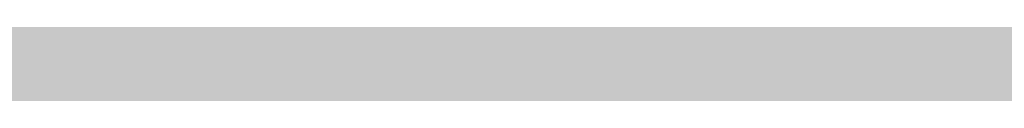
# Model space of a CAD drawing. Units: millimetres. Extents: x 0 to 2267, y 0 to 1823.
# Tile 178 of 256: x 1838.83 to 1841.442, y 1127.15 to 1127.306. Entities that reach past the tile are written whole.
import ezdxf

# ---------------------------------------------------------------- set-up
doc = ezdxf.new("R2010")
doc.units = ezdxf.units.MM
doc.header["$MEASUREMENT"] = 0
doc.layers.add('M-DIMS', color=2, linetype='Continuous', lineweight=25)
doc.layers.add('M-HATC', color=252, linetype='Continuous', lineweight=18)
doc.styles.get("Standard").update_dxf_attribs({"font": 'arial.ttf'})
doc.dimstyles.get("Standard").update_dxf_attribs({"dimtxt": 7, "dimasz": 4, "dimexe": 0.18, "dimexo": 0.0625, "dimgap": 0.09, "dimtad": 0, "dimdec": 0, "dimzin": 0, "dimdsep": 46, "dimtxsty": 'Standard', "dimcen": 0.09, "dimadec": 0, "dimazin": 0, "dimtfac": 1, "dimtdec": 0, "dimtofl": 0, "dimtmove": 0, "dimatfit": 3, "dimfxl": 1, "dimtolj": 1, "dimtzin": 0, "dimarcsym": 0})

# ---------------------------------------------------------------- blocks, each defined once
blk = doc.blocks.new('*D1')
at = {"layer": 'Defpoints', "color": 0, "transparency": 16777216}
for p in [(1593.4289, 1127.4171), (1843.4289, 1127.4171), (1843.4289, 955.6278)]:
    blk.add_point(p, dxfattribs=at)
at = {"layer": 'M-DIMS', "color": 0, "lineweight": -2, "transparency": 16777216}
for p, q in [((1593.4289, 1127.3546), (1593.4289, 955.4478)), ((1843.4289, 1127.3546), (1843.4289, 955.4478)), ((1597.4289, 955.6278), (1710.5582, 955.6278)), ((1839.4289, 955.6278), (1726.2996, 955.6278))]:
    blk.add_line(p, q, dxfattribs=at)
at = {"layer": 'M-DIMS', "color": 0, "transparency": 16777216}
for points in [[(1597.4289, 956.2944), (1597.4289, 954.9611), (1593.4289, 955.6278)], [(1839.4289, 956.2944), (1839.4289, 954.9611), (1843.4289, 955.6278)]]:
    blk.add_solid(points, dxfattribs=at)
at = {"layer": 'M-DIMS', "color": 0, "transparency": 16777216, "insert": (1718.4289, 955.6278), "char_height": 7, "attachment_point": 5}
blk.add_mtext('\\A1;250', dxfattribs=at)

msp = doc.modelspace()

# ---------------------------------------------------------------- hatches: boundary and pattern name
at = {"layer": 'M-HATC'}
h = msp.add_hatch(color=256, dxfattribs=at)
h.dxf.hatch_style = 1
h.paths.add_polyline_path([(2055.771, 1603.062), (1381.0868, 1603.062), (1381.0868, 1598.062), (2055.771, 1598.062)])
h.paths.add_polyline_path([(2055.771, 1598.062), (1381.0868, 1598.062), (1381.0868, 1593.062), (2055.771, 1593.062)])
h.paths.add_polyline_path([(2051.3074, 1536.7609), (1385.5504, 1536.7609), (1385.5504, 1526.7609), (1387.5504, 1526.7609), (1388.5366, 1525.0528), (1385.3319, 1521.2335), (1385.3319, 1521.2226), (2050.2542, 1522.7491), (2048.3212, 1525.0528), (2049.3074, 1526.7609), (2051.3074, 1526.7609)])
edge = h.paths.add_edge_path()
edge.add_arc((1847.5345, 1379.1492), 135, 222.603061, 222.890851, ccw=False)
edge.add_line((1748.1663, 1287.7656), (1683.0921, 1287.7656))
edge.add_arc((1583.7239, 1379.1492), 135, 317.109149, 317.396939, ccw=False)
edge.add_arc((1678.9686, 1290.6707), 5, 222.8909, 317.1091, ccw=False)
edge.add_arc((1774.2133, 1379.1492), 135, 222.603061, 222.890851, ccw=False)
edge.add_line((1674.8451, 1287.7656), (1609.7709, 1287.7656))
edge.add_arc((1510.4027, 1379.1492), 135, 317.109149, 317.396939, ccw=False)
edge.add_arc((1605.6474, 1290.6707), 5, 222.8909, 317.1091, ccw=False)
edge.add_arc((1700.8921, 1379.1492), 135, 222.603061, 222.890851, ccw=False)
edge.add_line((1601.5239, 1287.7656), (1536.4497, 1287.7656))
edge.add_arc((1437.0815, 1379.1492), 135, 317.109149, 317.396939, ccw=False)
edge.add_arc((1532.3262, 1290.6707), 5, 222.8909, 317.1091, ccw=False)
edge.add_arc((1627.5709, 1379.1492), 135, 222.603061, 222.890851, ccw=False)
edge.add_line((1528.2027, 1287.7656), (1505.9289, 1287.7656))
edge.add_spline(control_points=[(1505.9289, 1287.7656), (1504.2622, 1287.7656), (1504.2622, 1282.7656), (1505.9289, 1282.7656)], knot_values=[0, 0, 0, 0, 5, 5, 5, 5], degree=3, periodic=0)
edge.add_line((1505.9289, 1282.7656), (1930.9289, 1282.7656))
edge.add_spline(control_points=[(1930.9289, 1282.7656), (1932.5956, 1282.7656), (1932.5956, 1287.7656), (1930.9289, 1287.7656)], knot_values=[0, 0, 0, 0, 5, 5, 5, 5], degree=3, periodic=0)
edge.add_line((1930.9289, 1287.7656), (1903.0557, 1287.7656))
edge.add_arc((1803.6875, 1379.1492), 135, 317.109149, 317.396939, ccw=False)
edge.add_arc((1898.9322, 1290.6707), 5, 222.8909, 317.1091, ccw=False)
edge.add_arc((1994.1769, 1379.1492), 135, 222.603061, 222.890851, ccw=False)
edge.add_line((1894.8087, 1287.7656), (1829.7345, 1287.7656))
edge.add_arc((1730.3663, 1379.1492), 135, 317.109149, 317.396939, ccw=False)
edge.add_arc((1825.611, 1290.6707), 5, 222.8909, 317.1091, ccw=False)
edge.add_arc((1920.8557, 1379.1492), 135, 222.603061, 222.890851, ccw=False)
edge.add_line((1821.4875, 1287.7656), (1756.4133, 1287.7656))
edge.add_arc((1657.0451, 1379.1492), 135, 317.109149, 317.396939, ccw=False)
edge.add_arc((1752.2898, 1290.6707), 5, 222.8909, 317.1091, ccw=False)
edge = h.paths.add_edge_path()
edge.add_spline(control_points=[(1843.4289, 1227.2475), (1845.0956, 1227.2475), (1845.0956, 1232.2475), (1843.4289, 1232.2475)], knot_values=[0, 0, 0, 0, 5, 5, 5, 5], degree=3, periodic=0)
edge.add_line((1843.4289, 1232.2475), (1593.4289, 1232.2475))
edge.add_spline(control_points=[(1593.4289, 1232.2475), (1591.7622, 1232.2475), (1591.7622, 1227.2475), (1593.4289, 1227.2475)], knot_values=[0, 0, 0, 0, 5, 5, 5, 5], degree=3, periodic=0)
edge.add_line((1593.4289, 1227.2475), (1843.4289, 1227.2475))
h.paths.add_polyline_path([(1905.9289, 1127.4171), (1530.9289, 1127.4171, 0.414214), (1520.9289, 1117.4171), (1530.9289, 1117.4171), (1915.9289, 1117.4171, 0.414214)])
edge = h.paths.add_edge_path()
edge.add_arc((1397.0858, 1498.4078), 12.7299, 90.78215, 190.87871, ccw=False)
edge.add_line((1396.912, 1511.1365), (1428.0097, 1511.3488))
edge.add_line((1428.0097, 1511.3488), (1433.0097, 1511.3488))
edge.add_line((1433.0097, 1511.3488), (1434.439, 1511.3488))
edge.add_arc((1419.474, 1498.0804), 20, 41.561, 74.08211)
edge.add_line((1424.9592, 1517.3135), (1399.9351, 1517.2561))
edge.add_spline(control_points=[(1399.9307, 1517.2561), (1399.884, 1517.2131), (1399.8328, 1517.1689), (1399.7774, 1517.1236)], knot_values=[11.567499, 11.567499, 11.567499, 11.567499, 11.814249, 11.814249, 11.814249, 11.814249], degree=3, periodic=0)
edge.add_spline(control_points=[(1399.6328, 1517.0099), (1399.5831, 1516.9721), (1399.5307, 1516.9338), (1399.4759, 1516.8947)], knot_values=[11.167718, 11.167718, 11.167718, 11.167718, 11.365188, 11.365188, 11.365188, 11.365188], degree=3, periodic=0)
edge.add_spline(control_points=[(1399.3398, 1516.8001), (1399.1514, 1516.6719), (1398.9384, 1516.5377), (1398.704, 1516.3994)], knot_values=[10.376405, 10.376405, 10.376405, 10.376405, 11.00994, 11.00994, 11.00994, 11.00994], degree=3, periodic=0)
edge.add_spline(control_points=[(1398.6572, 1516.3719), (1398.5789, 1516.326), (1398.4983, 1516.2797), (1398.4155, 1516.2331)], knot_values=[10.125175, 10.125175, 10.125175, 10.125175, 10.334406, 10.334406, 10.334406, 10.334406], degree=3, periodic=0)
edge.add_spline(control_points=[(1398.2642, 1516.1487), (1398.196, 1516.1111), (1398.1263, 1516.0732), (1398.0555, 1516.0351)], knot_values=[9.832246, 9.832246, 9.832246, 9.832246, 9.999658, 9.999658, 9.999658, 9.999658], degree=3, periodic=0)
edge.add_spline(control_points=[(1397.9987, 1516.0048), (1397.7312, 1515.8621), (1397.446, 1515.7171), (1397.1466, 1515.5714)], knot_values=[9.161808, 9.161808, 9.161808, 9.161808, 9.787769, 9.787769, 9.787769, 9.787769], degree=3, periodic=0)
edge.add_spline(control_points=[(1397.1466, 1515.5714), (1396.8418, 1515.423), (1396.5222, 1515.274), (1396.1914, 1515.1262)], knot_values=[8.524455, 8.524455, 8.524455, 8.524455, 9.161808, 9.161808, 9.161808, 9.161808], degree=3, periodic=0)
edge.add_spline(control_points=[(1396.0777, 1515.0756), (1395.9854, 1515.0348), (1395.8922, 1514.994), (1395.7983, 1514.9534)], knot_values=[8.275193, 8.275193, 8.275193, 8.275193, 8.451726, 8.451726, 8.451726, 8.451726], degree=3, periodic=0)
edge.add_spline(control_points=[(1395.6018, 1514.8691), (1395.4997, 1514.8257), (1395.3968, 1514.7824), (1395.2932, 1514.7394)], knot_values=[7.962917, 7.962917, 7.962917, 7.962917, 8.152764, 8.152764, 8.152764, 8.152764], degree=3, periodic=0)
edge.add_spline(control_points=[(1395.2116, 1514.7057), (1394.8278, 1514.5475), (1394.4345, 1514.3929), (1394.0364, 1514.2442)], knot_values=[7.21254, 7.21254, 7.21254, 7.21254, 7.913148, 7.913148, 7.913148, 7.913148], degree=3, periodic=0)
edge.add_spline(control_points=[(1394.0364, 1514.2442), (1393.7076, 1514.1214), (1393.3754, 1514.0027), (1393.0427, 1513.8895)], knot_values=[6.633733, 6.633733, 6.633733, 6.633733, 7.21254, 7.21254, 7.21254, 7.21254], degree=3, periodic=0)
edge.add_spline(control_points=[(1392.8214, 1513.815), (1392.7198, 1513.7812), (1392.6181, 1513.7479), (1392.5166, 1513.7152)], knot_values=[6.328796, 6.328796, 6.328796, 6.328796, 6.505493, 6.505493, 6.505493, 6.505493], degree=3, periodic=0)
edge.add_spline(control_points=[(1392.5166, 1513.7152), (1392.3187, 1513.6515), (1392.1212, 1513.59), (1391.9244, 1513.531)], knot_values=[5.984605, 5.984605, 5.984605, 5.984605, 6.328796, 6.328796, 6.328796, 6.328796], degree=3, periodic=0)
edge.add_spline(control_points=[(1391.7915, 1513.4915), (1391.3122, 1513.3501), (1390.8384, 1513.2239), (1390.3784, 1513.1171)], knot_values=[5.066697, 5.066697, 5.066697, 5.066697, 5.907055, 5.907055, 5.907055, 5.907055], degree=3, periodic=0)
edge.add_spline(control_points=[(1390.3784, 1513.1171), (1390.1797, 1513.071), (1389.9836, 1513.0284), (1389.7907, 1512.9899)], knot_values=[4.70367, 4.70367, 4.70367, 4.70367, 5.066695, 5.066695, 5.066695, 5.066695], degree=3, periodic=0)
edge.add_spline(control_points=[(1389.422, 1512.9204), (1389.2459, 1512.8892), (1389.0729, 1512.8617), (1388.9036, 1512.8381)], knot_values=[4.130571, 4.130571, 4.130571, 4.130571, 4.469816, 4.469816, 4.469816, 4.469816], degree=3, periodic=0)
edge.add_spline(control_points=[(1388.9036, 1512.8381), (1388.591, 1512.7946), (1388.2911, 1512.7644), (1388.0071, 1512.7494)], knot_values=[3.504031, 3.504031, 3.504031, 3.504031, 4.130571, 4.130571, 4.130571, 4.130571], degree=3, periodic=0)
edge.add_spline(control_points=[(1387.9356, 1512.7459), (1387.8538, 1512.7423), (1387.7733, 1512.74), (1387.6944, 1512.739)], knot_values=[3.268866, 3.268866, 3.268866, 3.268866, 3.451164, 3.451164, 3.451164, 3.451164], degree=3, periodic=0)
edge.add_spline(control_points=[(1387.3351, 1512.7443), (1387.2076, 1512.7499), (1387.0847, 1512.7597), (1386.967, 1512.7739)], knot_values=[2.670686, 2.670686, 2.670686, 2.670686, 2.984, 2.984, 2.984, 2.984], degree=3, periodic=0)
edge.add_spline(control_points=[(1386.8327, 1512.7922), (1386.8209, 1512.7941), (1386.8092, 1512.7959), (1386.7975, 1512.7979)], knot_values=[2.516981, 2.516981, 2.516981, 2.516981, 2.549528, 2.549528, 2.549528, 2.549528], degree=3, periodic=0)
edge.add_spline(control_points=[(1386.4526, 1512.8735), (1386.4257, 1512.881), (1386.3993, 1512.889), (1386.3733, 1512.8972)], knot_values=[2.095869, 2.095869, 2.095869, 2.095869, 2.17941, 2.17941, 2.17941, 2.17941], degree=3, periodic=0)
edge.add_spline(control_points=[(1386.0691, 1513.0189), (1386.0634, 1513.0217), (1386.0577, 1513.0246), (1386.052, 1513.0275)], knot_values=[1.72453, 1.72453, 1.72453, 1.72453, 1.745933, 1.745933, 1.745933, 1.745933], degree=3, periodic=0)
edge.add_arc((1399.474, 1498.0804), 20, 131.82432, 180)
edge.add_arc((1630.3336, 1505.5484), 250.9708, 181.705176, 236.427975)
edge.add_arc((1605.3399, 1483.3044), 218.7822, 238.660829, 243.34961)
edge.add_arc((1647.0911, 1510.3592), 262.8986, 183.129836, 237.853442, ccw=False)
h.paths.add_polyline_path([(1406.5369, 1391.9644, 0.149382), (1491.5506, 1296.4418, -0.129517)], flags=17)
edge = h.paths.add_edge_path()
edge.add_arc((2037.3838, 1498.0804), 20, 0, 48.26587)
edge.add_spline(control_points=[(2050.6973, 1513.0052), (2050.6512, 1512.9847), (2050.6034, 1512.9655), (2050.5539, 1512.9477)], knot_values=[1.835652, 1.835652, 1.835652, 1.835652, 2.000781, 2.000781, 2.000781, 2.000781], degree=3, periodic=0)
edge.add_spline(control_points=[(2050.4616, 1512.9166), (2050.479, 1512.9221), (2050.4963, 1512.9277), (2050.5133, 1512.9335)], knot_values=[2.045477, 2.045477, 2.045477, 2.045477, 2.101389, 2.101389, 2.101389, 2.101389], degree=3, periodic=0)
edge.add_spline(control_points=[(2050.129, 1512.8342), (2050.1984, 1512.8473), (2050.2657, 1512.8623), (2050.3308, 1512.8792)], knot_values=[2.237629, 2.237629, 2.237629, 2.237629, 2.435841, 2.435841, 2.435841, 2.435841], degree=3, periodic=0)
edge.add_spline(control_points=[(2050.0946, 1512.8278), (2050.1061, 1512.8299), (2050.1176, 1512.832), (2050.129, 1512.8342)], knot_values=[2.435841, 2.435841, 2.435841, 2.435841, 2.468321, 2.468321, 2.468321, 2.468321], degree=3, periodic=0)
edge.add_spline(control_points=[(2049.7843, 1512.7851), (2049.8552, 1512.7922), (2049.9243, 1512.8008), (2049.9917, 1512.8109)], knot_values=[2.563852, 2.563852, 2.563852, 2.563852, 2.748541, 2.748541, 2.748541, 2.748541], degree=3, periodic=0)
edge.add_spline(control_points=[(2049.4052, 1512.7617), (2049.5364, 1512.7653), (2049.6629, 1512.773), (2049.7843, 1512.7851)], knot_values=[2.748541, 2.748541, 2.748541, 2.748541, 3.064882, 3.064882, 3.064882, 3.064882], degree=3, periodic=0)
edge.add_spline(control_points=[(2049.1698, 1512.7597), (2049.2336, 1512.7591), (2049.2965, 1512.7594), (2049.3584, 1512.7606)], knot_values=[3.102309, 3.102309, 3.102309, 3.102309, 3.2503, 3.2503, 3.2503, 3.2503], degree=3, periodic=0)
edge.add_spline(control_points=[(2048.8573, 1512.7691), (2048.9638, 1512.7638), (2049.068, 1512.7606), (2049.1698, 1512.7597)], knot_values=[3.2503, 3.2503, 3.2503, 3.2503, 3.486069, 3.486069, 3.486069, 3.486069], degree=3, periodic=0)
edge.add_spline(control_points=[(2048.6924, 1512.7789), (2048.3729, 1512.8009), (2048.0345, 1512.8411), (2047.6817, 1512.897)], knot_values=[3.606429, 3.606429, 3.606429, 3.606429, 4.2989, 4.2989, 4.2989, 4.2989], degree=3, periodic=0)
edge.add_spline(control_points=[(2047.6817, 1512.897), (2047.5458, 1512.9185), (2047.4077, 1512.9424), (2047.2678, 1512.9685)], knot_values=[4.2989, 4.2989, 4.2989, 4.2989, 4.565769, 4.565769, 4.565769, 4.565769], degree=3, periodic=0)
edge.add_spline(control_points=[(2047.2678, 1512.9685), (2047.1449, 1512.9914), (2047.0207, 1513.016), (2046.8951, 1513.0422)], knot_values=[4.565769, 4.565769, 4.565769, 4.565769, 4.799971, 4.799971, 4.799971, 4.799971], degree=3, periodic=0)
edge.add_spline(control_points=[(2046.8951, 1513.0422), (2046.5286, 1513.1188), (2046.1513, 1513.209), (2045.7676, 1513.3107)], knot_values=[4.799971, 4.799971, 4.799971, 4.799971, 5.483718, 5.483718, 5.483718, 5.483718], degree=3, periodic=0)
edge.add_spline(control_points=[(2045.7676, 1513.3107), (2045.3724, 1513.4154), (2044.9704, 1513.5322), (2044.5662, 1513.6588)], knot_values=[5.483718, 5.483718, 5.483718, 5.483718, 6.187866, 6.187866, 6.187866, 6.187866], degree=3, periodic=0)
edge.add_spline(control_points=[(2044.5662, 1513.6588), (2044.4149, 1513.7061), (2044.2633, 1513.7549), (2044.1116, 1513.8048)], knot_values=[6.187866, 6.187866, 6.187866, 6.187866, 6.451551, 6.451551, 6.451551, 6.451551], degree=3, periodic=0)
edge.add_spline(control_points=[(2044.1116, 1513.8048), (2043.9967, 1513.8427), (2043.8817, 1513.8813), (2043.7668, 1513.9205)], knot_values=[6.451551, 6.451551, 6.451551, 6.451551, 6.651434, 6.651434, 6.651434, 6.651434], degree=3, periodic=0)
edge.add_spline(control_points=[(2043.7668, 1513.9205), (2043.3716, 1514.0554), (2042.9774, 1514.1979), (2042.5886, 1514.3458)], knot_values=[6.651434, 6.651434, 6.651434, 6.651434, 7.338879, 7.338879, 7.338879, 7.338879], degree=3, periodic=0)
edge.add_spline(control_points=[(2042.5886, 1514.3458), (2042.1643, 1514.5071), (2041.7465, 1514.6749), (2041.3409, 1514.846)], knot_values=[7.338879, 7.338879, 7.338879, 7.338879, 8.089209, 8.089209, 8.089209, 8.089209], degree=3, periodic=0)
edge.add_spline(control_points=[(2041.3409, 1514.846), (2041.1028, 1514.9465), (2040.869, 1515.0481), (2040.6405, 1515.1502)], knot_values=[8.089209, 8.089209, 8.089209, 8.089209, 8.529587, 8.529587, 8.529587, 8.529587], degree=3, periodic=0)
edge.add_spline(control_points=[(2040.51, 1515.2089), (2040.0824, 1515.4022), (2039.6747, 1515.5971), (2039.295, 1515.7894)], knot_values=[8.613818, 8.613818, 8.613818, 8.613818, 9.44571, 9.44571, 9.44571, 9.44571], degree=3, periodic=0)
edge.add_spline(control_points=[(2039.295, 1515.7894), (2039.0618, 1515.9075), (2038.8391, 1516.0246), (2038.6288, 1516.1398)], knot_values=[9.44571, 9.44571, 9.44571, 9.44571, 9.956404, 9.956404, 9.956404, 9.956404], degree=3, periodic=0)
edge.add_spline(control_points=[(2038.6288, 1516.1398), (2038.5187, 1516.2001), (2038.4121, 1516.2598), (2038.309, 1516.3189)], knot_values=[9.956404, 9.956404, 9.956404, 9.956404, 10.223542, 10.223542, 10.223542, 10.223542], degree=3, periodic=0)
edge.add_spline(control_points=[(2038.309, 1516.3189), (2038.2138, 1516.3735), (2038.1216, 1516.4276), (2038.0328, 1516.481)], knot_values=[10.223542, 10.223542, 10.223542, 10.223542, 10.47051, 10.47051, 10.47051, 10.47051], degree=3, periodic=0)
edge.add_spline(control_points=[(2038.0328, 1516.481), (2037.7855, 1516.6296), (2037.5639, 1516.773), (2037.3722, 1516.909)], knot_values=[10.47051, 10.47051, 10.47051, 10.47051, 11.15767, 11.15767, 11.15767, 11.15767], degree=3, periodic=0)
edge.add_spline(control_points=[(2037.3722, 1516.909), (2037.2789, 1516.9752), (2037.1927, 1517.0396), (2037.1142, 1517.102)], knot_values=[11.15767, 11.15767, 11.15767, 11.15767, 11.49227, 11.49227, 11.49227, 11.49227], degree=3, periodic=0)
edge.add_spline(control_points=[(2036.8564, 1517.3259), (2036.9148, 1517.2692), (2036.9814, 1517.2103), (2037.0557, 1517.1492)], knot_values=[11.577341, 11.577341, 11.577341, 11.577341, 11.91035, 11.91035, 11.91035, 11.91035], degree=3, periodic=0)
edge.add_spline(control_points=[(2036.8074, 1517.3748), (2036.823, 1517.3587), (2036.8393, 1517.3424), (2036.8564, 1517.3259)], knot_values=[11.91035, 11.91035, 11.91035, 11.91035, 12.007402, 12.007402, 12.007402, 12.007402], degree=3, periodic=0)
edge.add_spline(control_points=[(2036.7017, 1517.494), (2036.7104, 1517.483), (2036.7196, 1517.4719), (2036.7291, 1517.4606)], knot_values=[12.184155, 12.184155, 12.184155, 12.184155, 12.255409, 12.255409, 12.255409, 12.255409], degree=3, periodic=0)
edge.add_spline(control_points=[(2036.6159, 1517.6205), (2036.62, 1517.613), (2036.6243, 1517.6055), (2036.6289, 1517.5979)], knot_values=[12.487913, 12.487913, 12.487913, 12.487913, 12.541035, 12.541035, 12.541035, 12.541035], degree=3, periodic=0)
edge.add_spline(control_points=[(2036.5635, 1517.786), (2036.5637, 1517.7794), (2036.5642, 1517.7726), (2036.565, 1517.7658)], knot_values=[12.911761, 12.911761, 12.911761, 12.911761, 12.968286, 12.968286, 12.968286, 12.968286], degree=3, periodic=0)
edge.add_spline(control_points=[(2036.6166, 1517.9304), (2036.6125, 1517.9259), (2036.6086, 1517.9212), (2036.6049, 1517.9165)], knot_values=[13.382527, 13.382527, 13.382527, 13.382527, 13.433791, 13.433791, 13.433791, 13.433791], degree=3, periodic=0)
edge.add_spline(control_points=[(2036.749, 1518.017), (2036.7361, 1518.0116), (2036.7239, 1518.006), (2036.7124, 1518.0002)], knot_values=[13.726299, 13.726299, 13.726299, 13.726299, 13.809928, 13.809928, 13.809928, 13.809928], degree=3, periodic=0)
edge.add_spline(control_points=[(2036.8604, 1518.0528), (2036.8386, 1518.0474), (2036.8181, 1518.0416), (2036.7988, 1518.0353)], knot_values=[13.910887, 13.910887, 13.910887, 13.910887, 14.02153, 14.02153, 14.02153, 14.02153], degree=3, periodic=0)
edge.add_line((2036.9639, 1518.0804), (2032.3838, 1518.0804))
edge.add_line((2032.3838, 1518.0804), (2027.3838, 1518.0804))
edge.add_line((2027.3838, 1518.0804), (2022.3838, 1518.0804))
edge.add_line((2022.3838, 1518.0804), (2017.3838, 1518.0804))
edge.add_arc((2017.3838, 1498.0804), 20, 90, 138.439)
edge.add_line((2002.4188, 1511.3488), (2003.8481, 1511.3488))
edge.add_line((2003.8481, 1511.3488), (2008.8481, 1511.3488))
edge.add_line((2008.8481, 1511.3488), (2039.772, 1511.1377))
edge.add_arc((2039.772, 1498.4078), 12.7299, -10.87871, 90, ccw=False)
edge.add_arc((1789.7668, 1510.3592), 262.8986, 302.146558, 356.870164, ccw=False)
edge.add_arc((1831.5179, 1483.3044), 218.7822, 296.65039, 301.339171)
edge.add_arc((1806.5242, 1505.5484), 250.9708, 303.572025, 358.294824)
h.paths.add_polyline_path([(2030.321, 1391.9644, -0.129517), (1945.3072, 1296.4418, 0.149382)], flags=17)
edge = h.paths.add_edge_path()
edge.add_spline(control_points=[(2037.2464, 1518.0821), (2037.2898, 1518.081), (2037.3355, 1518.0804), (2037.3838, 1518.0804)], knot_values=[0.000012, 0.000012, 0.000012, 0.000012, 0.144754, 0.144754, 0.144754, 0.144754], degree=3, periodic=0)
edge.add_line((2037.3357, 1518.0804), (2037.0096, 1518.0804))
edge.add_spline(control_points=[(2037.0096, 1518.0804), (2036.9822, 1518.0768), (2036.956, 1518.0727), (2036.9312, 1518.0681)], knot_values=[14.13465, 14.13465, 14.13465, 14.13465, 14.247197, 14.247197, 14.247197, 14.247197], degree=3, periodic=0)
edge.add_spline(control_points=[(2036.9312, 1518.0681), (2036.9276, 1518.0674), (2036.9241, 1518.0667), (2036.9205, 1518.0661)], knot_values=[14.118315, 14.118315, 14.118315, 14.118315, 14.13465, 14.13465, 14.13465, 14.13465], degree=3, periodic=0)
edge.add_spline(control_points=[(2036.9205, 1518.0661), (2036.9118, 1518.0644), (2036.9032, 1518.0626), (2036.8948, 1518.0608)], knot_values=[14.078086, 14.078086, 14.078086, 14.078086, 14.118315, 14.118315, 14.118315, 14.118315], degree=3, periodic=0)
edge.add_spline(control_points=[(2036.8948, 1518.0608), (2036.883, 1518.0583), (2036.8716, 1518.0556), (2036.8604, 1518.0528)], knot_values=[14.02153, 14.02153, 14.02153, 14.02153, 14.078086, 14.078086, 14.078086, 14.078086], degree=3, periodic=0)
edge.add_spline(control_points=[(2036.8604, 1518.0528), (2036.8386, 1518.0474), (2036.8181, 1518.0416), (2036.7988, 1518.0353)], knot_values=[13.910887, 13.910887, 13.910887, 13.910887, 14.02153, 14.02153, 14.02153, 14.02153], degree=3, periodic=0)
edge.add_spline(control_points=[(2036.7988, 1518.0353), (2036.7981, 1518.035), (2036.7974, 1518.0348), (2036.7967, 1518.0346)], knot_values=[13.906906, 13.906906, 13.906906, 13.906906, 13.910887, 13.910887, 13.910887, 13.910887], degree=3, periodic=0)
edge.add_spline(control_points=[(2036.7967, 1518.0346), (2036.7882, 1518.0318), (2036.7799, 1518.0289), (2036.7719, 1518.0259)], knot_values=[13.857826, 13.857826, 13.857826, 13.857826, 13.906906, 13.906906, 13.906906, 13.906906], degree=3, periodic=0)
edge.add_spline(control_points=[(2036.7719, 1518.0259), (2036.764, 1518.023), (2036.7564, 1518.02), (2036.749, 1518.017)], knot_values=[13.809928, 13.809928, 13.809928, 13.809928, 13.857826, 13.857826, 13.857826, 13.857826], degree=3, periodic=0)
edge.add_spline(control_points=[(2036.749, 1518.017), (2036.7361, 1518.0116), (2036.7239, 1518.006), (2036.7124, 1518.0002)], knot_values=[13.726299, 13.726299, 13.726299, 13.726299, 13.809928, 13.809928, 13.809928, 13.809928], degree=3, periodic=0)
edge.add_spline(control_points=[(2036.7124, 1518.0002), (2036.7121, 1518), (2036.7118, 1517.9999), (2036.7115, 1517.9997)], knot_values=[13.723993, 13.723993, 13.723993, 13.723993, 13.726299, 13.726299, 13.726299, 13.726299], degree=3, periodic=0)
edge.add_spline(control_points=[(2036.7115, 1517.9997), (2036.7063, 1517.9971), (2036.7013, 1517.9944), (2036.6965, 1517.9917)], knot_values=[13.686536, 13.686536, 13.686536, 13.686536, 13.723993, 13.723993, 13.723993, 13.723993], degree=3, periodic=0)
edge.add_spline(control_points=[(2036.6965, 1517.9917), (2036.6919, 1517.9891), (2036.6874, 1517.9865), (2036.6831, 1517.9839)], knot_values=[13.651251, 13.651251, 13.651251, 13.651251, 13.686536, 13.686536, 13.686536, 13.686536], degree=3, periodic=0)
edge.add_spline(control_points=[(2036.6831, 1517.9839), (2036.6764, 1517.9798), (2036.67, 1517.9757), (2036.6639, 1517.9714)], knot_values=[13.596804, 13.596804, 13.596804, 13.596804, 13.651251, 13.651251, 13.651251, 13.651251], degree=3, periodic=0)
edge.add_spline(control_points=[(2036.6639, 1517.9714), (2036.6636, 1517.9712), (2036.6633, 1517.9709), (2036.6629, 1517.9707)], knot_values=[13.593956, 13.593956, 13.593956, 13.593956, 13.596804, 13.596804, 13.596804, 13.596804], degree=3, periodic=0)
edge.add_spline(control_points=[(2036.6629, 1517.9707), (2036.6603, 1517.9689), (2036.6577, 1517.967), (2036.6552, 1517.9651)], knot_values=[13.570322, 13.570322, 13.570322, 13.570322, 13.593956, 13.593956, 13.593956, 13.593956], degree=3, periodic=0)
edge.add_spline(control_points=[(2036.6552, 1517.9651), (2036.6525, 1517.9631), (2036.6499, 1517.9611), (2036.6474, 1517.9591)], knot_values=[13.545477, 13.545477, 13.545477, 13.545477, 13.570322, 13.570322, 13.570322, 13.570322], degree=3, periodic=0)
edge.add_spline(control_points=[(2036.6474, 1517.9591), (2036.6472, 1517.9589), (2036.6471, 1517.9588), (2036.6469, 1517.9587)], knot_values=[13.543931, 13.543931, 13.543931, 13.543931, 13.545477, 13.545477, 13.545477, 13.545477], degree=3, periodic=0)
edge.add_spline(control_points=[(2036.6469, 1517.9587), (2036.6412, 1517.9541), (2036.6358, 1517.9494), (2036.6307, 1517.9447)], knot_values=[13.488237, 13.488237, 13.488237, 13.488237, 13.543931, 13.543931, 13.543931, 13.543931], degree=3, periodic=0)
edge.add_spline(control_points=[(2036.6307, 1517.9447), (2036.6282, 1517.9423), (2036.6257, 1517.9399), (2036.6233, 1517.9374)], knot_values=[13.460307, 13.460307, 13.460307, 13.460307, 13.488237, 13.488237, 13.488237, 13.488237], degree=3, periodic=0)
edge.add_spline(control_points=[(2036.6233, 1517.9374), (2036.6215, 1517.9356), (2036.6198, 1517.9338), (2036.6181, 1517.932)], knot_values=[13.439712, 13.439712, 13.439712, 13.439712, 13.460307, 13.460307, 13.460307, 13.460307], degree=3, periodic=0)
edge.add_spline(control_points=[(2036.6181, 1517.932), (2036.6176, 1517.9315), (2036.6171, 1517.9309), (2036.6166, 1517.9304)], knot_values=[13.433791, 13.433791, 13.433791, 13.433791, 13.439712, 13.439712, 13.439712, 13.439712], degree=3, periodic=0)
edge.add_spline(control_points=[(2036.6166, 1517.9304), (2036.6125, 1517.9259), (2036.6086, 1517.9212), (2036.6049, 1517.9165)], knot_values=[13.382527, 13.382527, 13.382527, 13.382527, 13.433791, 13.433791, 13.433791, 13.433791], degree=3, periodic=0)
edge.add_spline(control_points=[(2036.6049, 1517.9165), (2036.6026, 1517.9135), (2036.6004, 1517.9104), (2036.5982, 1517.9074)], knot_values=[13.350017, 13.350017, 13.350017, 13.350017, 13.382527, 13.382527, 13.382527, 13.382527], degree=3, periodic=0)
edge.add_spline(control_points=[(2036.5982, 1517.9074), (2036.5972, 1517.9059), (2036.5962, 1517.9043), (2036.5952, 1517.9028)], knot_values=[13.333922, 13.333922, 13.333922, 13.333922, 13.350017, 13.350017, 13.350017, 13.350017], degree=3, periodic=0)
edge.add_spline(control_points=[(2036.5952, 1517.9028), (2036.5945, 1517.9018), (2036.5939, 1517.9009), (2036.5933, 1517.8999)], knot_values=[13.323828, 13.323828, 13.323828, 13.323828, 13.333922, 13.333922, 13.333922, 13.333922], degree=3, periodic=0)
edge.add_spline(control_points=[(2036.5933, 1517.8999), (2036.5905, 1517.8955), (2036.5879, 1517.8909), (2036.5855, 1517.8864)], knot_values=[13.277545, 13.277545, 13.277545, 13.277545, 13.323828, 13.323828, 13.323828, 13.323828], degree=3, periodic=0)
edge.add_spline(control_points=[(2036.5855, 1517.8864), (2036.5836, 1517.8827), (2036.5817, 1517.8789), (2036.5801, 1517.8751)], knot_values=[13.240119, 13.240119, 13.240119, 13.240119, 13.277545, 13.277545, 13.277545, 13.277545], degree=3, periodic=0)
edge.add_spline(control_points=[(2036.5801, 1517.8751), (2036.5795, 1517.8739), (2036.579, 1517.8727), (2036.5785, 1517.8715)], knot_values=[13.228211, 13.228211, 13.228211, 13.228211, 13.240119, 13.240119, 13.240119, 13.240119], degree=3, periodic=0)
edge.add_spline(control_points=[(2036.5785, 1517.8715), (2036.578, 1517.8702), (2036.5774, 1517.869), (2036.5769, 1517.8677)], knot_values=[13.215717, 13.215717, 13.215717, 13.215717, 13.228211, 13.228211, 13.228211, 13.228211], degree=3, periodic=0)
edge.add_spline(control_points=[(2036.5769, 1517.8677), (2036.5755, 1517.864), (2036.5741, 1517.8603), (2036.5729, 1517.8565)], knot_values=[13.179847, 13.179847, 13.179847, 13.179847, 13.215717, 13.215717, 13.215717, 13.215717], degree=3, periodic=0)
edge.add_spline(control_points=[(2036.5729, 1517.8565), (2036.5713, 1517.8515), (2036.5699, 1517.8464), (2036.5687, 1517.8413)], knot_values=[13.132017, 13.132017, 13.132017, 13.132017, 13.179847, 13.179847, 13.179847, 13.179847], degree=3, periodic=0)
edge.add_spline(control_points=[(2036.5687, 1517.8413), (2036.5684, 1517.8402), (2036.5682, 1517.8392), (2036.568, 1517.8382)], knot_values=[13.122482, 13.122482, 13.122482, 13.122482, 13.132017, 13.132017, 13.132017, 13.132017], degree=3, periodic=0)
edge.add_spline(control_points=[(2036.568, 1517.8382), (2036.5676, 1517.8363), (2036.5672, 1517.8345), (2036.5669, 1517.8327)], knot_values=[13.105592, 13.105592, 13.105592, 13.105592, 13.122482, 13.122482, 13.122482, 13.122482], degree=3, periodic=0)
edge.add_spline(control_points=[(2036.5669, 1517.8327), (2036.5662, 1517.8292), (2036.5657, 1517.8257), (2036.5652, 1517.8222)], knot_values=[13.074063, 13.074063, 13.074063, 13.074063, 13.105592, 13.105592, 13.105592, 13.105592], degree=3, periodic=0)
edge.add_spline(control_points=[(2036.5652, 1517.8222), (2036.5652, 1517.8222), (2036.5652, 1517.8222), (2036.5652, 1517.8222)], knot_values=[13.074043, 13.074043, 13.074043, 13.074043, 13.074063, 13.074063, 13.074063, 13.074063], degree=3, periodic=0)
edge.add_spline(control_points=[(2036.5652, 1517.8222), (2036.5644, 1517.8164), (2036.5639, 1517.8106), (2036.5636, 1517.8046)], knot_values=[13.021884, 13.021884, 13.021884, 13.021884, 13.074043, 13.074043, 13.074043, 13.074043], degree=3, periodic=0)
edge.add_spline(control_points=[(2036.5636, 1517.8046), (2036.5636, 1517.804), (2036.5636, 1517.8034), (2036.5635, 1517.8028)], knot_values=[13.01674, 13.01674, 13.01674, 13.01674, 13.021884, 13.021884, 13.021884, 13.021884], degree=3, periodic=0)
edge.add_spline(control_points=[(2036.5635, 1517.8028), (2036.5634, 1517.8005), (2036.5634, 1517.7982), (2036.5634, 1517.7958)], knot_values=[12.996438, 12.996438, 12.996438, 12.996438, 13.01674, 13.01674, 13.01674, 13.01674], degree=3, periodic=0)
edge.add_spline(control_points=[(2036.5634, 1517.7958), (2036.5633, 1517.7926), (2036.5634, 1517.7893), (2036.5635, 1517.786)], knot_values=[12.968286, 12.968286, 12.968286, 12.968286, 12.996438, 12.996438, 12.996438, 12.996438], degree=3, periodic=0)
edge.add_spline(control_points=[(2036.5635, 1517.786), (2036.5637, 1517.7794), (2036.5642, 1517.7726), (2036.565, 1517.7658)], knot_values=[12.911761, 12.911761, 12.911761, 12.911761, 12.968286, 12.968286, 12.968286, 12.968286], degree=3, periodic=0)
edge.add_spline(control_points=[(2036.565, 1517.7658), (2036.565, 1517.7657), (2036.565, 1517.7656), (2036.565, 1517.7656)], knot_values=[12.911017, 12.911017, 12.911017, 12.911017, 12.911761, 12.911761, 12.911761, 12.911761], degree=3, periodic=0)
edge.add_spline(control_points=[(2036.565, 1517.7656), (2036.5654, 1517.7625), (2036.5658, 1517.7593), (2036.5663, 1517.7562)], knot_values=[12.88528, 12.88528, 12.88528, 12.88528, 12.911017, 12.911017, 12.911017, 12.911017], degree=3, periodic=0)
edge.add_spline(control_points=[(2036.5663, 1517.7562), (2036.5667, 1517.7534), (2036.5672, 1517.7506), (2036.5677, 1517.7478)], knot_values=[12.862519, 12.862519, 12.862519, 12.862519, 12.88528, 12.88528, 12.88528, 12.88528], degree=3, periodic=0)
edge.add_spline(control_points=[(2036.5677, 1517.7478), (2036.5678, 1517.7474), (2036.5679, 1517.7469), (2036.568, 1517.7465)], knot_values=[12.858885, 12.858885, 12.858885, 12.858885, 12.862519, 12.862519, 12.862519, 12.862519], degree=3, periodic=0)
edge.add_spline(control_points=[(2036.568, 1517.7465), (2036.5692, 1517.7399), (2036.5707, 1517.7332), (2036.5724, 1517.7264)], knot_values=[12.8053, 12.8053, 12.8053, 12.8053, 12.858885, 12.858885, 12.858885, 12.858885], degree=3, periodic=0)
edge.add_spline(control_points=[(2036.5724, 1517.7264), (2036.5734, 1517.7226), (2036.5745, 1517.7187), (2036.5756, 1517.7149)], knot_values=[12.775176, 12.775176, 12.775176, 12.775176, 12.8053, 12.8053, 12.8053, 12.8053], degree=3, periodic=0)
edge.add_spline(control_points=[(2036.5756, 1517.7149), (2036.5763, 1517.7125), (2036.577, 1517.7102), (2036.5778, 1517.7078)], knot_values=[12.756759, 12.756759, 12.756759, 12.756759, 12.775176, 12.775176, 12.775176, 12.775176], degree=3, periodic=0)
edge.add_spline(control_points=[(2036.5778, 1517.7078), (2036.5781, 1517.7067), (2036.5784, 1517.7057), (2036.5787, 1517.7047)], knot_values=[12.748742, 12.748742, 12.748742, 12.748742, 12.756759, 12.756759, 12.756759, 12.756759], degree=3, periodic=0)
edge.add_spline(control_points=[(2036.5787, 1517.7047), (2036.5808, 1517.6983), (2036.5831, 1517.6919), (2036.5856, 1517.6854)], knot_values=[12.69959, 12.69959, 12.69959, 12.69959, 12.748742, 12.748742, 12.748742, 12.748742], degree=3, periodic=0)
edge.add_spline(control_points=[(2036.5856, 1517.6854), (2036.5876, 1517.68), (2036.5898, 1517.6746), (2036.5921, 1517.6692)], knot_values=[12.659038, 12.659038, 12.659038, 12.659038, 12.69959, 12.69959, 12.69959, 12.69959], degree=3, periodic=0)
edge.add_spline(control_points=[(2036.5921, 1517.6692), (2036.594, 1517.6648), (2036.5959, 1517.6605), (2036.5979, 1517.6561)], knot_values=[12.626806, 12.626806, 12.626806, 12.626806, 12.659038, 12.659038, 12.659038, 12.659038], degree=3, periodic=0)
edge.add_spline(control_points=[(2036.5979, 1517.6561), (2036.5984, 1517.6551), (2036.5989, 1517.6541), (2036.5993, 1517.6531)], knot_values=[12.619394, 12.619394, 12.619394, 12.619394, 12.626806, 12.626806, 12.626806, 12.626806], degree=3, periodic=0)
edge.add_spline(control_points=[(2036.5993, 1517.6531), (2036.6043, 1517.6424), (2036.6099, 1517.6315), (2036.6159, 1517.6205)], knot_values=[12.541039, 12.541039, 12.541039, 12.541039, 12.619394, 12.619394, 12.619394, 12.619394], degree=3, periodic=0)
edge.add_spline(control_points=[(2036.6159, 1517.6205), (2036.6159, 1517.6205), (2036.6159, 1517.6205), (2036.6159, 1517.6205)], knot_values=[12.541035, 12.541035, 12.541035, 12.541035, 12.541039, 12.541039, 12.541039, 12.541039], degree=3, periodic=0)
edge.add_spline(control_points=[(2036.6159, 1517.6205), (2036.62, 1517.613), (2036.6243, 1517.6055), (2036.6289, 1517.5979)], knot_values=[12.487913, 12.487913, 12.487913, 12.487913, 12.541035, 12.541035, 12.541035, 12.541035], degree=3, periodic=0)
edge.add_spline(control_points=[(2036.6289, 1517.5979), (2036.6326, 1517.5916), (2036.6365, 1517.5853), (2036.6406, 1517.5789)], knot_values=[12.443982, 12.443982, 12.443982, 12.443982, 12.487913, 12.487913, 12.487913, 12.487913], degree=3, periodic=0)
edge.add_spline(control_points=[(2036.6406, 1517.5789), (2036.6414, 1517.5776), (2036.6423, 1517.5763), (2036.6431, 1517.5749)], knot_values=[12.434996, 12.434996, 12.434996, 12.434996, 12.443982, 12.443982, 12.443982, 12.443982], degree=3, periodic=0)
edge.add_spline(control_points=[(2036.6431, 1517.5749), (2036.6531, 1517.5596), (2036.6639, 1517.5439), (2036.6756, 1517.528)], knot_values=[12.329647, 12.329647, 12.329647, 12.329647, 12.434996, 12.434996, 12.434996, 12.434996], degree=3, periodic=0)
edge.add_spline(control_points=[(2036.6756, 1517.528), (2036.6839, 1517.5168), (2036.6925, 1517.5055), (2036.7017, 1517.494)], knot_values=[12.255409, 12.255409, 12.255409, 12.255409, 12.329647, 12.329647, 12.329647, 12.329647], degree=3, periodic=0)
edge.add_spline(control_points=[(2036.7017, 1517.494), (2036.7104, 1517.483), (2036.7196, 1517.4719), (2036.7291, 1517.4606)], knot_values=[12.184155, 12.184155, 12.184155, 12.184155, 12.255409, 12.255409, 12.255409, 12.255409], degree=3, periodic=0)
edge.add_spline(control_points=[(2036.7291, 1517.4606), (2036.7436, 1517.4435), (2036.759, 1517.4262), (2036.7753, 1517.4085)], knot_values=[12.075961, 12.075961, 12.075961, 12.075961, 12.184155, 12.184155, 12.184155, 12.184155], degree=3, periodic=0)
edge.add_spline(control_points=[(2036.7753, 1517.4085), (2036.7763, 1517.4075), (2036.7773, 1517.4064), (2036.7783, 1517.4054)], knot_values=[12.069502, 12.069502, 12.069502, 12.069502, 12.075961, 12.075961, 12.075961, 12.075961], degree=3, periodic=0)
edge.add_spline(control_points=[(2036.7783, 1517.4054), (2036.7877, 1517.3953), (2036.7974, 1517.385), (2036.8074, 1517.3748)], knot_values=[12.007402, 12.007402, 12.007402, 12.007402, 12.069502, 12.069502, 12.069502, 12.069502], degree=3, periodic=0)
edge.add_spline(control_points=[(2036.8074, 1517.3748), (2036.823, 1517.3587), (2036.8393, 1517.3424), (2036.8564, 1517.3259)], knot_values=[11.91035, 11.91035, 11.91035, 11.91035, 12.007402, 12.007402, 12.007402, 12.007402], degree=3, periodic=0)
edge.add_spline(control_points=[(2036.8564, 1517.3259), (2036.9148, 1517.2692), (2036.9814, 1517.2103), (2037.0557, 1517.1492)], knot_values=[11.577341, 11.577341, 11.577341, 11.577341, 11.91035, 11.91035, 11.91035, 11.91035], degree=3, periodic=0)
edge.add_spline(control_points=[(2037.0557, 1517.1492), (2037.0747, 1517.1336), (2037.0942, 1517.1179), (2037.1142, 1517.102)], knot_values=[11.49227, 11.49227, 11.49227, 11.49227, 11.577341, 11.577341, 11.577341, 11.577341], degree=3, periodic=0)
edge.add_spline(control_points=[(2037.1142, 1517.102), (2037.1927, 1517.0396), (2037.2789, 1516.9752), (2037.3722, 1516.909)], knot_values=[11.15767, 11.15767, 11.15767, 11.15767, 11.49227, 11.49227, 11.49227, 11.49227], degree=3, periodic=0)
edge.add_spline(control_points=[(2037.3722, 1516.909), (2037.5639, 1516.773), (2037.7855, 1516.6296), (2038.0328, 1516.481)], knot_values=[10.47051, 10.47051, 10.47051, 10.47051, 11.15767, 11.15767, 11.15767, 11.15767], degree=3, periodic=0)
edge.add_spline(control_points=[(2038.0328, 1516.481), (2038.1216, 1516.4276), (2038.2138, 1516.3735), (2038.309, 1516.3189)], knot_values=[10.223542, 10.223542, 10.223542, 10.223542, 10.47051, 10.47051, 10.47051, 10.47051], degree=3, periodic=0)
edge.add_spline(control_points=[(2038.309, 1516.3189), (2038.4121, 1516.2598), (2038.5187, 1516.2001), (2038.6288, 1516.1398)], knot_values=[9.956404, 9.956404, 9.956404, 9.956404, 10.223542, 10.223542, 10.223542, 10.223542], degree=3, periodic=0)
edge.add_spline(control_points=[(2038.6288, 1516.1398), (2038.8391, 1516.0246), (2039.0618, 1515.9075), (2039.295, 1515.7894)], knot_values=[9.44571, 9.44571, 9.44571, 9.44571, 9.956404, 9.956404, 9.956404, 9.956404], degree=3, periodic=0)
edge.add_spline(control_points=[(2039.295, 1515.7894), (2039.6747, 1515.5971), (2040.0824, 1515.4022), (2040.51, 1515.2089)], knot_values=[8.613818, 8.613818, 8.613818, 8.613818, 9.44571, 9.44571, 9.44571, 9.44571], degree=3, periodic=0)
edge.add_spline(control_points=[(2040.51, 1515.2089), (2040.5533, 1515.1893), (2040.5968, 1515.1697), (2040.6405, 1515.1502)], knot_values=[8.529587, 8.529587, 8.529587, 8.529587, 8.613818, 8.613818, 8.613818, 8.613818], degree=3, periodic=0)
edge.add_spline(control_points=[(2040.6405, 1515.1502), (2040.869, 1515.0481), (2041.1028, 1514.9465), (2041.3409, 1514.846)], knot_values=[8.089209, 8.089209, 8.089209, 8.089209, 8.529587, 8.529587, 8.529587, 8.529587], degree=3, periodic=0)
edge.add_spline(control_points=[(2041.3409, 1514.846), (2041.7465, 1514.6749), (2042.1643, 1514.5071), (2042.5886, 1514.3458)], knot_values=[7.338879, 7.338879, 7.338879, 7.338879, 8.089209, 8.089209, 8.089209, 8.089209], degree=3, periodic=0)
edge.add_spline(control_points=[(2042.5886, 1514.3458), (2042.9774, 1514.1979), (2043.3716, 1514.0554), (2043.7668, 1513.9205)], knot_values=[6.651434, 6.651434, 6.651434, 6.651434, 7.338879, 7.338879, 7.338879, 7.338879], degree=3, periodic=0)
edge.add_spline(control_points=[(2043.7668, 1513.9205), (2043.8817, 1513.8813), (2043.9967, 1513.8427), (2044.1116, 1513.8048)], knot_values=[6.451551, 6.451551, 6.451551, 6.451551, 6.651434, 6.651434, 6.651434, 6.651434], degree=3, periodic=0)
edge.add_spline(control_points=[(2044.1116, 1513.8048), (2044.2633, 1513.7549), (2044.4149, 1513.7061), (2044.5662, 1513.6588)], knot_values=[6.187866, 6.187866, 6.187866, 6.187866, 6.451551, 6.451551, 6.451551, 6.451551], degree=3, periodic=0)
edge.add_spline(control_points=[(2044.5662, 1513.6588), (2044.9704, 1513.5322), (2045.3724, 1513.4154), (2045.7676, 1513.3107)], knot_values=[5.483718, 5.483718, 5.483718, 5.483718, 6.187866, 6.187866, 6.187866, 6.187866], degree=3, periodic=0)
edge.add_spline(control_points=[(2045.7676, 1513.3107), (2046.1513, 1513.209), (2046.5286, 1513.1188), (2046.8951, 1513.0422)], knot_values=[4.799971, 4.799971, 4.799971, 4.799971, 5.483718, 5.483718, 5.483718, 5.483718], degree=3, periodic=0)
edge.add_spline(control_points=[(2046.8951, 1513.0422), (2047.0207, 1513.016), (2047.1449, 1512.9914), (2047.2678, 1512.9685)], knot_values=[4.565769, 4.565769, 4.565769, 4.565769, 4.799971, 4.799971, 4.799971, 4.799971], degree=3, periodic=0)
edge.add_spline(control_points=[(2047.2678, 1512.9685), (2047.4077, 1512.9424), (2047.5458, 1512.9185), (2047.6817, 1512.897)], knot_values=[4.2989, 4.2989, 4.2989, 4.2989, 4.565769, 4.565769, 4.565769, 4.565769], degree=3, periodic=0)
edge.add_spline(control_points=[(2047.6817, 1512.897), (2048.0345, 1512.8411), (2048.3729, 1512.8009), (2048.6924, 1512.7789)], knot_values=[3.606429, 3.606429, 3.606429, 3.606429, 4.2989, 4.2989, 4.2989, 4.2989], degree=3, periodic=0)
edge.add_spline(control_points=[(2048.6924, 1512.7789), (2048.7479, 1512.7751), (2048.8029, 1512.7718), (2048.8573, 1512.7691)], knot_values=[3.486069, 3.486069, 3.486069, 3.486069, 3.606429, 3.606429, 3.606429, 3.606429], degree=3, periodic=0)
edge.add_spline(control_points=[(2048.8573, 1512.7691), (2048.9638, 1512.7638), (2049.068, 1512.7606), (2049.1698, 1512.7597)], knot_values=[3.2503, 3.2503, 3.2503, 3.2503, 3.486069, 3.486069, 3.486069, 3.486069], degree=3, periodic=0)
edge.add_spline(control_points=[(2049.1698, 1512.7597), (2049.2336, 1512.7591), (2049.2965, 1512.7594), (2049.3584, 1512.7606)], knot_values=[3.102309, 3.102309, 3.102309, 3.102309, 3.2503, 3.2503, 3.2503, 3.2503], degree=3, periodic=0)
edge.add_spline(control_points=[(2049.3584, 1512.7606), (2049.3741, 1512.7609), (2049.3897, 1512.7613), (2049.4052, 1512.7617)], knot_values=[3.064882, 3.064882, 3.064882, 3.064882, 3.102309, 3.102309, 3.102309, 3.102309], degree=3, periodic=0)
edge.add_spline(control_points=[(2049.4052, 1512.7617), (2049.5364, 1512.7653), (2049.6629, 1512.773), (2049.7843, 1512.7851)], knot_values=[2.748541, 2.748541, 2.748541, 2.748541, 3.064882, 3.064882, 3.064882, 3.064882], degree=3, periodic=0)
edge.add_spline(control_points=[(2049.7843, 1512.7851), (2049.8552, 1512.7922), (2049.9243, 1512.8008), (2049.9917, 1512.8109)], knot_values=[2.563852, 2.563852, 2.563852, 2.563852, 2.748541, 2.748541, 2.748541, 2.748541], degree=3, periodic=0)
edge.add_spline(control_points=[(2049.9917, 1512.8109), (2050.0265, 1512.8161), (2050.0608, 1512.8218), (2050.0946, 1512.8278)], knot_values=[2.468321, 2.468321, 2.468321, 2.468321, 2.563852, 2.563852, 2.563852, 2.563852], degree=3, periodic=0)
edge.add_spline(control_points=[(2050.0946, 1512.8278), (2050.1061, 1512.8299), (2050.1176, 1512.832), (2050.129, 1512.8342)], knot_values=[2.435841, 2.435841, 2.435841, 2.435841, 2.468321, 2.468321, 2.468321, 2.468321], degree=3, periodic=0)
edge.add_spline(control_points=[(2050.129, 1512.8342), (2050.1984, 1512.8473), (2050.2657, 1512.8623), (2050.3308, 1512.8792)], knot_values=[2.237629, 2.237629, 2.237629, 2.237629, 2.435841, 2.435841, 2.435841, 2.435841], degree=3, periodic=0)
edge.add_spline(control_points=[(2050.3308, 1512.8792), (2050.3754, 1512.8908), (2050.4191, 1512.9032), (2050.4616, 1512.9166)], knot_values=[2.101389, 2.101389, 2.101389, 2.101389, 2.237629, 2.237629, 2.237629, 2.237629], degree=3, periodic=0)
edge.add_spline(control_points=[(2050.4616, 1512.9166), (2050.479, 1512.9221), (2050.4963, 1512.9277), (2050.5133, 1512.9335)], knot_values=[2.045477, 2.045477, 2.045477, 2.045477, 2.101389, 2.101389, 2.101389, 2.101389], degree=3, periodic=0)
edge.add_spline(control_points=[(2050.5133, 1512.9335), (2050.527, 1512.9382), (2050.5405, 1512.9429), (2050.5539, 1512.9477)], knot_values=[2.000781, 2.000781, 2.000781, 2.000781, 2.045477, 2.045477, 2.045477, 2.045477], degree=3, periodic=0)
edge.add_spline(control_points=[(2050.5539, 1512.9477), (2050.6034, 1512.9655), (2050.6512, 1512.9847), (2050.6973, 1513.0052)], knot_values=[1.835652, 1.835652, 1.835652, 1.835652, 2.000781, 2.000781, 2.000781, 2.000781], degree=3, periodic=0)
edge.add_arc((2037.3838, 1498.0804), 20, 48.26587, 90.12993)
edge = h.paths.add_edge_path(flags=16)
edge.add_spline(control_points=[(1386.1389, 1512.9859), (1388.92, 1511.7395), (1398.0387, 1515.5187), (1399.9307, 1517.2561)], knot_values=[1.831046, 1.831046, 1.831046, 1.831046, 11.814249, 11.814249, 11.814249, 11.814249], degree=3, periodic=0)
edge.add_line((1399.9307, 1517.2561), (1393.7435, 1517.2419))
edge.add_arc((1399.474, 1498.0804), 20, 106.6501, 131.8173)

# ---------------------------------------------------------------- dimensions: what is measured, and where the dimension line sits
at = {"layer": 'M-DIMS'}
dim = msp.add_linear_dim(base=(1843.4289, 955.6278), p1=(1593.4289, 1127.4171), p2=(1843.4289, 1127.4171), dimstyle='Standard', override={"dimclrd": 0, "dimclre": 0, "dimclrt": 0}, dxfattribs=at)
dim.commit()
dim.dimension.update_dxf_attribs({"geometry": '*D1', "text_midpoint": (1718.4289, 955.6278)})

doc.saveas('drawing.dxf')
